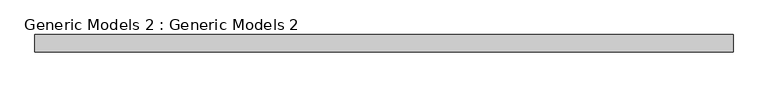
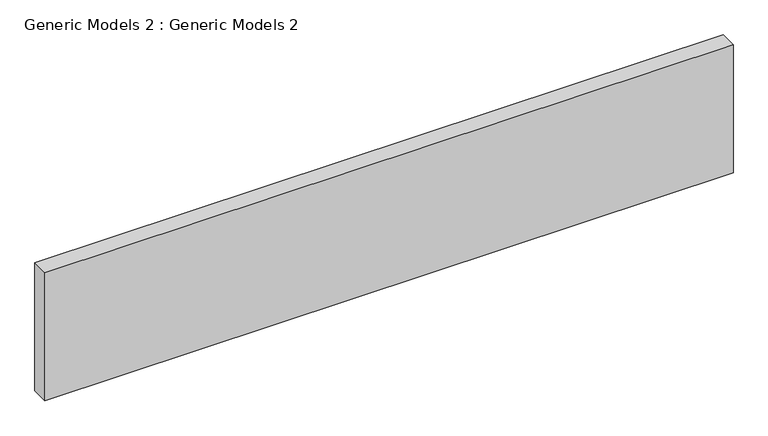
"""IFC4 building model written with IfcOpenShell, lengths in millimetres: proxy geometry, Generic Models 2 : Generic Models 2."""

from ifc_helpers import new_model, si_unit, frame, origin, place, context, project, spatial, polyline, outline, extrude, source, transform, mapped, element, save


def generic_models_2_generic_models_2_90455f6d(model_context):
    return source(origin(), model_context, "Body", "SweptSolid", [
        extrude(outline(polyline([(2724.9503979, -6558.2938352), (-3366.5453131, -6558.2938352), (-3366.5453131, -6405.8938352), (2724.9503979, -6405.8938352), (2724.9503979, -6558.2938352)])), frame((0.0, 0.0, 3352.8), z_axis=(0.0, 0.0, 1.0), x_axis=(1.0, 0.0, 0.0)), (0.0, 0.0, 1.0), 1197.560949),
    ])


if __name__ == "__main__":
    model = new_model("IFC4")
    model_context = context("Model", 3, world=origin())
    ifc_project = project(units=[si_unit("LENGTHUNIT", "METRE", prefix="MILLI")], contexts=[model_context])
    site = spatial("IfcSite", under=ifc_project)
    building = spatial("IfcBuilding", under=site)
    placement = place(None, origin())
    generic_models_2_generic_models_2_shape = generic_models_2_generic_models_2_90455f6d(model_context)
    element("IfcBuildingElementProxy", 1, Name="Generic Models 2 : Generic Models 2", ObjectType="Generic Models 2 : Generic Models 2", at=placement, inside=building, context=model_context, shape_type="MappedRepresentation", body=[
        mapped(generic_models_2_generic_models_2_shape, transform((0.0, 0.0, 0.0), x_axis=(1.0, 0.0, 0.0), y_axis=(0.0, 1.0, 0.0), z_axis=(0.0, 0.0, 1.0))),
    ])
    save(model, "model.ifc")

# Revit data of these elements
# Element 1 (IfcBuildingElementProxy, "Generic Models 2 : Generic Models 2")
#   Materials on its faces: "WALL PAINT"
# Materials
#   "WALL PAINT": class "Generic", colour RGB 120 120 120, transparency 0, Cost = 0
